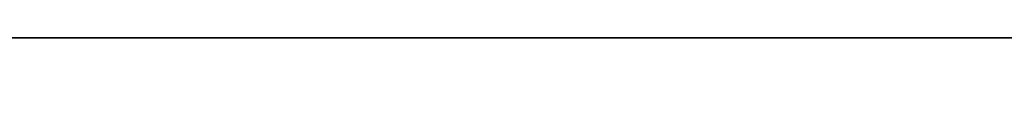
# Model space of a CAD drawing. Units: inches. Extents: x -86 to 2463, y -1058 to 68.
# Tile 6 of 17: x 32 to 49, y -304 to -303. Entities that reach past the tile are written whole.
import ezdxf

# ---------------------------------------------------------------- set-up
doc = ezdxf.new("R2010")
doc.units = ezdxf.units.IN
doc.header["$MEASUREMENT"] = 0
doc.layers.add('A-ANNO-DIMS', color=2, linetype='Continuous', lineweight=18)
doc.layers.add('A-WALL', color=7, linetype='Continuous', lineweight=35)
doc.styles.get("Standard").update_dxf_attribs({"font": 'arial.ttf'})
doc.dimstyles.get("Standard").update_dxf_attribs({"dimtxt": 0.18, "dimasz": 0.18, "dimexe": 0.18, "dimexo": 0.0625, "dimgap": 0.09, "dimtad": 0, "dimtih": 1, "dimtoh": 1, "dimdec": 4, "dimzin": 0, "dimdsep": 46, "dimtxsty": 'Standard', "dimcen": 0.09, "dimadec": 0, "dimazin": 0, "dimtfac": 1, "dimtdec": 4, "dimtofl": 0, "dimtmove": 0, "dimatfit": 3, "dimfxl": 1, "dimtolj": 1, "dimtzin": 0, "dimarcsym": 0})

# ---------------------------------------------------------------- blocks, each defined once
blk = doc.blocks.new('*D41')
at = {"layer": 'A-ANNO-DIMS', "color": 0, "lineweight": -2, "transparency": 16777216}
for p, q in [((15.761, -303.167), (15.761, -740.384)), ((68.889, -303.167), (68.889, -740.384)), ((15.941, -740.204), (41.931, -740.204)), ((68.709, -740.204), (42.719, -740.204))]:
    blk.add_line(p, q, dxfattribs=at)
at = {"layer": 'A-ANNO-DIMS', "color": 0, "transparency": 16777216}
for points in [[(15.941, -740.174), (15.941, -740.234), (15.761, -740.204)], [(68.709, -740.174), (68.709, -740.234), (68.889, -740.204)]]:
    blk.add_solid(points, dxfattribs=at)
at = {"layer": 'Defpoints', "color": 0, "transparency": 16777216}
for p in [(15.761, -303.104), (68.889, -303.104), (68.889, -740.204)]:
    blk.add_point(p, dxfattribs=at)
at = {"layer": 'A-ANNO-DIMS', "color": 0, "transparency": 16777216, "insert": (42.325, -740.204), "char_height": 0.18, "attachment_point": 5}
blk.add_mtext('\\A1;53.13', dxfattribs=at)

msp = doc.modelspace()

# ---------------------------------------------------------------- linework, layer by layer
at = {"layer": 'A-WALL'}
msp.add_line((377.846, -303.104), (15.761, -303.104), dxfattribs=at)

# ---------------------------------------------------------------- dimensions: what is measured, and where the dimension line sits
at = {"layer": 'A-ANNO-DIMS'}
dim = msp.add_linear_dim(base=(68.889, -740.204), p1=(15.761, -303.104), p2=(68.889, -303.104), dimstyle='Standard', override={"dimdec": 2, "dimlfac": 1, "dimrnd": 0, "dimzin": 0, "dimdsep": 46, "dimlunit": 2}, dxfattribs=at)
dim.commit()
dim.dimension.update_dxf_attribs({"geometry": '*D41', "text_midpoint": (42.325, -740.204)})

doc.saveas('drawing.dxf')
